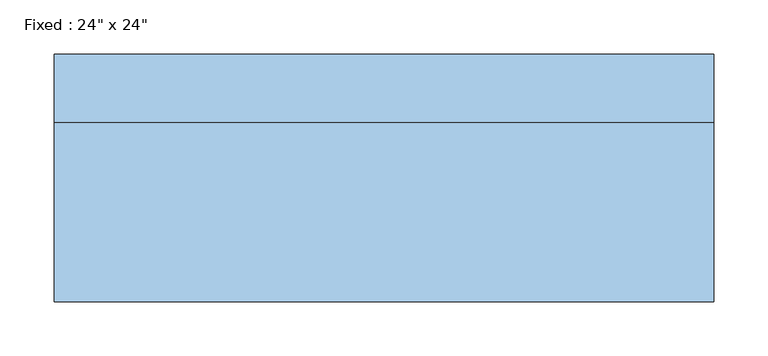
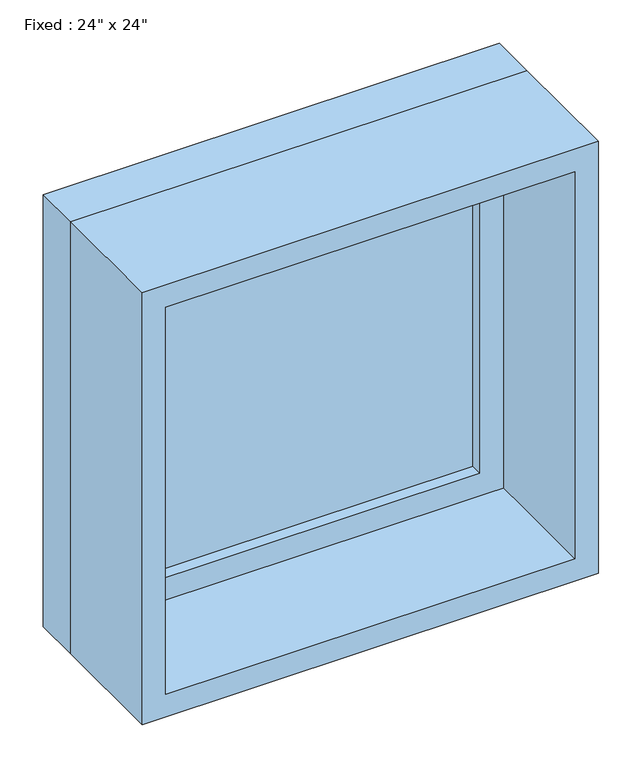
"""IFC4 building model written with IfcOpenShell, lengths in millimetres: window geometry."""

from ifc_helpers import new_model, si_unit, frame, origin, place, context, project, spatial, polyline, outline, extrude, source, transform, mapped, element, save


def window_80340324(model_context):
    return source(origin(), model_context, "Body", "SweptSolid", [
        extrude(outline(polyline([(203.2, 66.675), (-279.4, 66.675), (-279.4, 79.375), (203.2, 79.375), (203.2, 66.675)])), frame((0.0, 0.0, 977.9), z_axis=(0.0, 0.0, 1.0), x_axis=(1.0, 0.0, 0.0)), (0.0, 0.0, 1.0), 482.6),
        extrude(outline(polyline([(1504.95, -323.85), (933.45, -323.85), (933.45, 247.65), (1504.95, 247.65), (1504.95, -323.85)]), holes=[polyline([(1460.5, -279.4), (1460.5, 203.2), (977.9, 203.2), (977.9, -279.4), (1460.5, -279.4)])]), frame((0.0, 50.8, 0.0), z_axis=(0.0, 1.0, 0.0), x_axis=(0.0, 0.0, 1.0)), (0.0, 0.0, 1.0), 44.45),
        extrude(outline(polyline([(1524.0, -342.9), (914.4, -342.9), (914.4, 266.7), (1524.0, 266.7), (1524.0, -342.9)]), holes=[polyline([(1492.25, -311.15), (1492.25, 234.95), (946.15, 234.95), (946.15, -311.15), (1492.25, -311.15)])]), frame((0.0, -114.3, 0.0), z_axis=(0.0, 1.0, 0.0), x_axis=(0.0, 0.0, 1.0)), (0.0, 0.0, 1.0), 165.1),
        extrude(outline(polyline([(1524.0, 266.7), (1524.0, -342.9), (914.4, -342.9), (914.4, 266.7), (1524.0, 266.7)]), holes=[polyline([(1504.95, 247.65), (933.45, 247.65), (933.45, -323.85), (1504.95, -323.85), (1504.95, 247.65)])]), frame((0.0, 50.8, 0.0), z_axis=(0.0, 1.0, 0.0), x_axis=(0.0, 0.0, 1.0)), (0.0, 0.0, 1.0), 63.5),
    ])


if __name__ == "__main__":
    model = new_model("IFC4")
    model_context = context("Model", 3, world=origin())
    ifc_project = project(units=[si_unit("LENGTHUNIT", "METRE", prefix="MILLI")], contexts=[model_context])
    site = spatial("IfcSite", under=ifc_project)
    building = spatial("IfcBuilding", under=site)
    placement = place(None, origin())
    window_shape = window_80340324(model_context)
    element("IfcWindow", 1, ObjectType="Fixed : 24\" x 24\"", at=placement, inside=building, context=model_context, shape_type="MappedRepresentation", body=[
        mapped(window_shape, transform((0.0, 0.0, 0.0), x_axis=(1.0, 0.0, 0.0), y_axis=(0.0, 1.0, 0.0), z_axis=(0.0, 0.0, 1.0))),
    ])
    save(model, "model.ifc")

# Revit data of these elements
# Type "Fixed : 24\" x 24\""
#   Type Mark = "3"
#   Construction Type Id = "GSP4R"
#   Assembly Code = "B2020100"
#   Analytic Construction = "1/8 in Pilkington single glazing"
#   Visual Light Transmittance = 0.9
#   Solar Heat Gain Coefficient = 0.78
#   Heat Transfer Coefficient (U) = 0.6496 BTU/(h·ft²·°F)
#   Height = 2' - 0"
#   Default Sill Height = 3' - 0"
#   Width = 2' - 0"
#   Window Inset = 0' - 0 3/4"
#   Define Thermal Properties by = 1
#   Define Thermal Properties by = 1
#   Glass Pane Material = Glass
#   Sash Material = Sash
#   Wall Closure = (empty or 0)
# Element 1 (IfcWindow, "Fixed : 24\" x 24\"")
#   Materials on its faces: "Sash", "Glass"
# Materials
#   "Glass": class "Glass", colour RGB 0 128 192, transparency 0.75, Description = "Soda Lime Glass", Cost = 0
#   "Sash": class "Wood", colour RGB 224 178 126, transparency 0, Cost = 0
